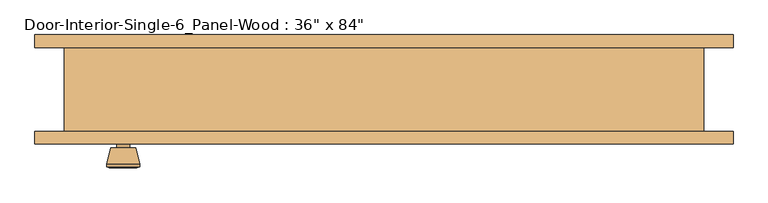
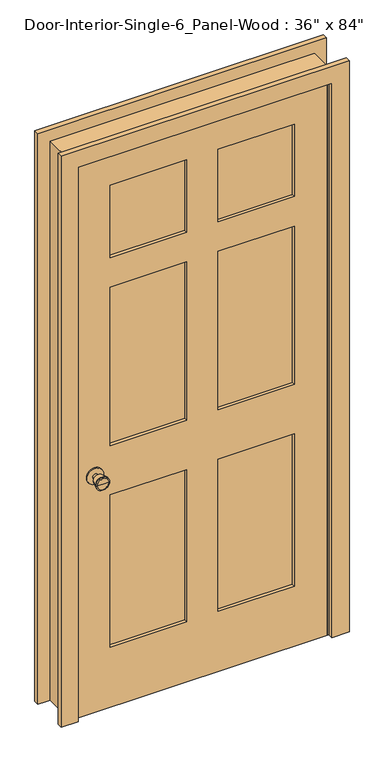
"""IFC4 building model written with IfcOpenShell, lengths in millimetres: door geometry."""

from ifc_helpers import new_model, si_unit, point, frame, frame_2d, origin, place, context, project, spatial, polyline, circle_curve, trimmed, segment, composite_curve, outline, extrude, faceted_brep, source, transform, mapped, element, save
from ifc_brep_helpers import plane_surface, cylinder_surface, revolved_surface, advanced_brep


def door_c610b25b(model_context):
    return source(origin(), model_context, "Body", "SolidModel", [
        advanced_brep(
        [(-393.7, -19.4, 914.4), (-403.7, -19.4, 914.4), (-383.7, -19.4, 914.4), (-373.2241324, 29.6, 914.4), (-414.1758676, 29.6, 914.4), (-393.7, 29.6, 914.4), (-368.7, 27.7721319, 914.4), (-418.7, 27.7721319, 914.4), (-368.7, 24.3084537, 914.4), (-418.7, 24.3084537, 914.4), (-375.063764, -0.4, 914.4), (-412.336236, -0.4, 914.4), (-383.7, -0.4, 914.4), (-403.7, -0.4, 914.4)],
        [
            (0, 1),
            (1, 2, circle_curve(frame((-393.7, -19.4, 914.4), z_axis=(0.0, -1.0, 0.0), x_axis=(-1.0, 0.0, 0.0)), 10.0)),
            (2, 0),
            (2, 1, circle_curve(frame((-393.7, -19.4, 914.4), z_axis=(0.0, -1.0, 0.0), x_axis=(-1.0, 0.0, 0.0)), 10.0)),
            (3, 4, circle_curve(frame((-393.7, 29.6, 914.4), z_axis=(0.0, 1.0, 0.0), x_axis=(-1.0, 0.0, 0.0)), 20.4758676)),
            (4, 5),
            (5, 3),
            (4, 3, circle_curve(frame((-393.7, 29.6, 914.4), z_axis=(0.0, 1.0, 0.0), x_axis=(-1.0, 0.0, 0.0)), 20.4758676)),
            (6, 7, circle_curve(frame((-393.7, 27.7721319, 914.4), z_axis=(0.0, 1.0, 0.0), x_axis=(-1.0, 0.0, 0.0)), 25.0)),
            (7, 4),
            (3, 6),
            (7, 6, circle_curve(frame((-393.7, 27.7721319, 914.4), z_axis=(0.0, 1.0, 0.0), x_axis=(-1.0, 0.0, 0.0)), 25.0)),
            (8, 9, circle_curve(frame((-393.7, 24.3084537, 914.4), z_axis=(0.0, 1.0, 0.0), x_axis=(-1.0, 0.0, 0.0)), 25.0)),
            (9, 7),
            (6, 8),
            (9, 8, circle_curve(frame((-393.7, 24.3084537, 914.4), z_axis=(0.0, 1.0, 0.0), x_axis=(-1.0, 0.0, 0.0)), 25.0)),
            (10, 11, circle_curve(frame((-393.7, -0.4, 914.4), z_axis=(0.0, 1.0, 0.0), x_axis=(-1.0, 0.0, 0.0)), 18.636236)),
            (11, 9),
            (8, 10),
            (11, 10, circle_curve(frame((-393.7, -0.4, 914.4), z_axis=(0.0, 1.0, 0.0), x_axis=(-1.0, 0.0, 0.0)), 18.636236)),
            (12, 13, circle_curve(frame((-393.7, -0.4, 914.4), z_axis=(0.0, 1.0, 0.0), x_axis=(-1.0, 0.0, 0.0)), 10.0)),
            (13, 11),
            (10, 12),
            (13, 12, circle_curve(frame((-393.7, -0.4, 914.4), z_axis=(0.0, 1.0, 0.0), x_axis=(-1.0, 0.0, 0.0)), 10.0)),
            (1, 13),
            (12, 2),
        ],
        [
            plane_surface(frame((-393.7, -19.4, 914.4), z_axis=(0.0, -1.0, 0.0), x_axis=(-1.0, 0.0, 0.0))),
            plane_surface(frame((-393.7, 29.6, 914.4), z_axis=(0.0, 1.0, 0.0), x_axis=(-1.0, 0.0, 0.0))),
            revolved_surface(polyline([(-414.1758676, 29.6, 914.4), (-418.7, 27.7721319, 914.4)]), (-393.7, -19.4, 914.4), (0.0, -1.0, 0.0)),
            cylinder_surface(frame((-393.7, -19.4, 914.4), z_axis=(0.0, -1.0, 0.0), x_axis=(-1.0, 0.0, 0.0)), 25.0),
            revolved_surface(polyline([(-418.7, 24.3084537, 914.4), (-412.336236, -0.4, 914.4)]), (-393.7, -19.4, 914.4), (0.0, -1.0, 0.0)),
            plane_surface(frame((-393.7, -0.4, 914.4), z_axis=(0.0, -1.0, 0.0), x_axis=(-1.0, 0.0, 0.0))),
            cylinder_surface(frame((-393.7, -19.4, 914.4), z_axis=(0.0, -1.0, 0.0), x_axis=(-1.0, 0.0, 0.0)), 10.0),
        ],
        [
            (0, [[1, 2, 3]]),
            (0, [[-3, 4, -1]]),
            (1, [[5, 6, 7]]),
            (1, [[8, -7, -6]]),
            (2, [[9, 10, -5, 11]]),
            (2, [[12, -11, -8, -10]]),
            (3, [[13, 14, -9, 15]]),
            (3, [[16, -15, -12, -14]]),
            (4, [[17, 18, -13, 19]]),
            (4, [[20, -19, -16, -18]]),
            (5, [[21, 22, -17, 23]]),
            (5, [[24, -23, -20, -22]]),
            (6, [[-2, 25, -21, 26]]),
            (6, [[-4, -26, -24, -25]]),
        ],
    ),
        extrude(outline(composite_curve([segment(trimmed(circle_curve(frame_2d((914.4, -393.7)), 30.0), [point((914.4, -423.7))], [point((914.4, -363.7))], False, "CARTESIAN"), True, "CONTINUOUS"), segment(trimmed(circle_curve(frame_2d((914.4, -393.7)), 30.0), [point((914.4, -363.7))], [point((914.4, -423.7))], False, "CARTESIAN"), True, "CONTINUOUS")], self_intersect=False)), frame((0.0, -25.4, 0.0), z_axis=(0.0, 1.0, 0.0), x_axis=(0.0, 0.0, 1.0)), (0.0, 0.0, 1.0), 6.0),
        advanced_brep(
        [(-393.7, -66.325, 914.4), (-383.7, -66.325, 914.4), (-403.7, -66.325, 914.4), (-373.2241324, -115.325, 914.4), (-393.7, -115.325, 914.4), (-414.1758676, -115.325, 914.4), (-368.7, -113.4971319, 914.4), (-418.7, -113.4971319, 914.4), (-368.7, -110.0334537, 914.4), (-418.7, -110.0334537, 914.4), (-375.063764, -85.325, 914.4), (-412.336236, -85.325, 914.4), (-383.7, -85.325, 914.4), (-403.7, -85.325, 914.4)],
        [
            (0, 1),
            (1, 2, circle_curve(frame((-393.7, -66.325, 914.4), z_axis=(0.0, 1.0, 0.0), x_axis=(-1.0, 0.0, 0.0)), 10.0)),
            (2, 0),
            (2, 1, circle_curve(frame((-393.7, -66.325, 914.4), z_axis=(0.0, 1.0, 0.0), x_axis=(-1.0, 0.0, 0.0)), 10.0)),
            (3, 4),
            (4, 5),
            (5, 3, circle_curve(frame((-393.7, -115.325, 914.4), z_axis=(0.0, -1.0, 0.0), x_axis=(-1.0, 0.0, 0.0)), 20.4758676)),
            (3, 5, circle_curve(frame((-393.7, -115.325, 914.4), z_axis=(0.0, -1.0, 0.0), x_axis=(-1.0, 0.0, 0.0)), 20.4758676)),
            (6, 3),
            (5, 7),
            (7, 6, circle_curve(frame((-393.7, -113.4971319, 914.4), z_axis=(0.0, -1.0, 0.0), x_axis=(-1.0, 0.0, 0.0)), 25.0)),
            (6, 7, circle_curve(frame((-393.7, -113.4971319, 914.4), z_axis=(0.0, -1.0, 0.0), x_axis=(-1.0, 0.0, 0.0)), 25.0)),
            (8, 6),
            (7, 9),
            (9, 8, circle_curve(frame((-393.7, -110.0334537, 914.4), z_axis=(0.0, -1.0, 0.0), x_axis=(-1.0, 0.0, 0.0)), 25.0)),
            (8, 9, circle_curve(frame((-393.7, -110.0334537, 914.4), z_axis=(0.0, -1.0, 0.0), x_axis=(-1.0, 0.0, 0.0)), 25.0)),
            (10, 8),
            (9, 11),
            (11, 10, circle_curve(frame((-393.7, -85.325, 914.4), z_axis=(0.0, -1.0, 0.0), x_axis=(-1.0, 0.0, 0.0)), 18.636236)),
            (10, 11, circle_curve(frame((-393.7, -85.325, 914.4), z_axis=(0.0, -1.0, 0.0), x_axis=(-1.0, 0.0, 0.0)), 18.636236)),
            (12, 10),
            (11, 13),
            (13, 12, circle_curve(frame((-393.7, -85.325, 914.4), z_axis=(0.0, -1.0, 0.0), x_axis=(-1.0, 0.0, 0.0)), 10.0)),
            (12, 13, circle_curve(frame((-393.7, -85.325, 914.4), z_axis=(0.0, -1.0, 0.0), x_axis=(-1.0, 0.0, 0.0)), 10.0)),
            (1, 12),
            (13, 2),
        ],
        [
            plane_surface(frame((-393.7, -66.325, 914.4), z_axis=(0.0, 1.0, 0.0), x_axis=(-1.0, 0.0, 0.0))),
            plane_surface(frame((-393.7, -115.325, 914.4), z_axis=(0.0, -1.0, 0.0), x_axis=(-1.0, 0.0, 0.0))),
            revolved_surface(polyline([(-414.1758676, -115.325, 914.4), (-418.7, -113.4971319, 914.4)]), (-393.7, -66.325, 914.4), (0.0, 1.0, 0.0)),
            cylinder_surface(frame((-393.7, -66.325, 914.4), z_axis=(0.0, 1.0, 0.0), x_axis=(-1.0, 0.0, 0.0)), 25.0),
            revolved_surface(polyline([(-418.7, -110.0334537, 914.4), (-412.336236, -85.325, 914.4)]), (-393.7, -66.325, 914.4), (0.0, 1.0, 0.0)),
            plane_surface(frame((-393.7, -85.325, 914.4), z_axis=(0.0, 1.0, 0.0), x_axis=(-1.0, 0.0, 0.0))),
            cylinder_surface(frame((-393.7, -66.325, 914.4), z_axis=(0.0, 1.0, 0.0), x_axis=(-1.0, 0.0, 0.0)), 10.0),
        ],
        [
            (0, [[1, 2, 3]]),
            (0, [[-3, 4, -1]]),
            (1, [[5, 6, 7]]),
            (1, [[-6, -5, 8]]),
            (2, [[9, -7, 10, 11]]),
            (2, [[-10, -8, -9, 12]]),
            (3, [[13, -11, 14, 15]]),
            (3, [[-14, -12, -13, 16]]),
            (4, [[17, -15, 18, 19]]),
            (4, [[-18, -16, -17, 20]]),
            (5, [[21, -19, 22, 23]]),
            (5, [[-22, -20, -21, 24]]),
            (6, [[25, -23, 26, -2]]),
            (6, [[-26, -24, -25, -4]]),
        ],
    ),
        extrude(outline(composite_curve([segment(trimmed(circle_curve(frame_2d((914.4, -393.7)), 30.0), [point((914.4, -423.7))], [point((914.4, -363.7))], False, "CARTESIAN"), True, "CONTINUOUS"), segment(trimmed(circle_curve(frame_2d((914.4, -393.7)), 30.0), [point((914.4, -363.7))], [point((914.4, -423.7))], False, "CARTESIAN"), True, "CONTINUOUS")], self_intersect=False)), frame((0.0, -66.325, 0.0), z_axis=(0.0, 1.0, 0.0), x_axis=(0.0, 0.0, 1.0)), (0.0, 0.0, 1.0), 6.0),
        faceted_brep([(482.6, -60.325, 0.0), (457.2, -60.325, 0.0), (457.2, -25.4, 0.0), (444.5, -25.4, 0.0), (444.5, 9.525, 0.0), (457.2, 9.525, 0.0), (457.2, 66.675, 0.0), (482.6, 66.675, 0.0), (482.6, 66.675, 2159.0), (482.6, -60.325, 2159.0), (457.2, 66.675, 2133.6), (-457.2, 66.675, 2133.6), (-457.2, 66.675, 0.0), (-482.6, 66.675, 0.0), (-482.6, 66.675, 2159.0), (457.2, 9.525, 2133.6), (444.5, 9.525, 2120.9), (-444.5, 9.525, 2120.9), (-444.5, 9.525, 0.0), (-457.2, 9.525, 0.0), (-457.2, 9.525, 2133.6), (444.5, -25.4, 2120.9), (457.2, -25.4, 2133.6), (-457.2, -25.4, 2133.6), (-457.2, -25.4, 0.0), (-444.5, -25.4, 0.0), (-444.5, -25.4, 2120.9), (457.2, -60.325, 2133.6), (-482.6, -60.325, 2159.0), (-482.6, -60.325, 0.0), (-457.2, -60.325, 0.0), (-457.2, -60.325, 2133.6)], [[[0, 1, 2, 3, 4, 5, 6, 7]], [[7, 8, 9, 0]], [[6, 10, 11, 12, 13, 14, 8, 7]], [[5, 15, 10, 6]], [[4, 16, 17, 18, 19, 20, 15, 5]], [[3, 21, 16, 4]], [[2, 22, 23, 24, 25, 26, 21, 3]], [[1, 27, 22, 2]], [[0, 9, 28, 29, 30, 31, 27, 1]], [[8, 14, 28, 9]], [[15, 20, 11, 10]], [[21, 26, 17, 16]], [[27, 31, 23, 22]], [[29, 13, 12, 19, 18, 25, 24, 30]], [[14, 13, 29, 28]], [[20, 19, 12, 11]], [[26, 25, 18, 17]], [[31, 30, 24, 23]]]),
        extrude(outline(polyline([(2133.6, -457.2), (0.0, -457.2), (0.0, 457.2), (2133.6, 457.2), (2133.6, -457.2)]), holes=[polyline([(2014.5375, 57.15), (2014.5375, 336.55), (1735.1375, 336.55), (1735.1375, 57.15), (2014.5375, 57.15)]), polyline([(1620.8375, 336.55), (1009.65, 336.55), (1009.65, 57.15), (1620.8375, 57.15), (1620.8375, 336.55)]), polyline([(1009.65, -57.15), (1009.65, -336.55), (1620.8375, -336.55), (1620.8375, -57.15), (1009.65, -57.15)]), polyline([(1735.1375, -336.55), (2014.5375, -336.55), (2014.5375, -57.15), (1735.1375, -57.15), (1735.1375, -336.55)]), polyline([(819.15, 57.15), (819.15, 336.55), (231.775, 336.55), (231.775, 57.15), (819.15, 57.15)]), polyline([(231.775, -57.15), (231.775, -336.55), (819.15, -336.55), (819.15, -57.15), (231.775, -57.15)])]), frame((0.0, -60.325, 0.0), z_axis=(0.0, 1.0, 0.0), x_axis=(0.0, 0.0, 1.0)), (0.0, 0.0, 1.0), 34.925),
        extrude(outline(polyline([(336.55, -37.0416667), (336.55, -48.6833333), (57.15, -48.6833333), (57.15, -37.0416667), (336.55, -37.0416667)])), frame((0.0, 0.0, 1735.1375), z_axis=(0.0, 0.0, 1.0), x_axis=(1.0, 0.0, 0.0)), (0.0, 0.0, 1.0), 279.4),
        extrude(outline(polyline([(336.55, -37.0416667), (336.55, -48.6833333), (57.15, -48.6833333), (57.15, -37.0416667), (336.55, -37.0416667)])), frame((0.0, 0.0, 1009.65), z_axis=(0.0, 0.0, 1.0), x_axis=(1.0, 0.0, 0.0)), (0.0, 0.0, 1.0), 611.1875),
        extrude(outline(polyline([(-57.15, -37.0416667), (-57.15, -48.6833333), (-336.55, -48.6833333), (-336.55, -37.0416667), (-57.15, -37.0416667)])), frame((0.0, 0.0, 1009.65), z_axis=(0.0, 0.0, 1.0), x_axis=(1.0, 0.0, 0.0)), (0.0, 0.0, 1.0), 611.1875),
        extrude(outline(polyline([(-57.15, -37.0416667), (-57.15, -48.6833333), (-336.55, -48.6833333), (-336.55, -37.0416667), (-57.15, -37.0416667)])), frame((0.0, 0.0, 1735.1375), z_axis=(0.0, 0.0, 1.0), x_axis=(1.0, 0.0, 0.0)), (0.0, 0.0, 1.0), 279.4),
        extrude(outline(polyline([(336.55, -37.0416667), (336.55, -48.6833333), (57.15, -48.6833333), (57.15, -37.0416667), (336.55, -37.0416667)])), frame((0.0, 0.0, 231.775), z_axis=(0.0, 0.0, 1.0), x_axis=(1.0, 0.0, 0.0)), (0.0, 0.0, 1.0), 587.375),
        extrude(outline(polyline([(-57.15, -37.0416667), (-57.15, -48.6833333), (-336.55, -48.6833333), (-336.55, -37.0416667), (-57.15, -37.0416667)])), frame((0.0, 0.0, 231.775), z_axis=(0.0, 0.0, 1.0), x_axis=(1.0, 0.0, 0.0)), (0.0, 0.0, 1.0), 587.375),
        extrude(outline(polyline([(0.0, 527.05), (2203.45, 527.05), (2203.45, -527.05), (0.0, -527.05), (0.0, -463.55), (2139.95, -463.55), (2139.95, 463.55), (0.0, 463.55), (0.0, 527.05)])), frame((0.0, -79.375, 0.0), z_axis=(0.0, 1.0, 0.0), x_axis=(0.0, 0.0, 1.0)), (0.0, 0.0, 1.0), 19.05),
        extrude(outline(polyline([(0.0, 527.05), (2203.45, 527.05), (2203.45, -527.05), (0.0, -527.05), (0.0, -463.55), (2139.95, -463.55), (2139.95, 463.55), (0.0, 463.55), (0.0, 527.05)])), frame((0.0, 66.675, 0.0), z_axis=(0.0, 1.0, 0.0), x_axis=(0.0, 0.0, 1.0)), (0.0, 0.0, 1.0), 19.05),
    ])


if __name__ == "__main__":
    model = new_model("IFC4")
    model_context = context("Model", 3, world=origin())
    ifc_project = project(units=[si_unit("LENGTHUNIT", "METRE", prefix="MILLI")], contexts=[model_context])
    site = spatial("IfcSite", under=ifc_project)
    building = spatial("IfcBuilding", under=site)
    placement = place(None, origin())
    door_shape = door_c610b25b(model_context)
    element("IfcDoor", 1, ObjectType="Door-Interior-Single-6_Panel-Wood : 36\" x 84\"", at=placement, inside=building, context=model_context, shape_type="MappedRepresentation", body=[
        mapped(door_shape, transform((0.0, 0.0, 0.0), x_axis=(1.0, 0.0, 0.0), y_axis=(0.0, 1.0, 0.0), z_axis=(0.0, 0.0, 1.0))),
    ])
    save(model, "model.ifc")

# Revit data of these elements
# Type "Door-Interior-Single-6_Panel-Wood : 36\" x 84\""
#   Type Mark = "12"
#   Assembly Code = "C1020300"
#   Analytic Construction = "Wooden"
#   Top Rail = 0' - 4 11/16"
#   Top Panel = 0' - 11"
#   Thickness = 0' - 1 3/8"
#   Thermal Resistance (R) = 2.5876 (h·ft²·°F)/BTU
#   Swing Angle [instance default] = 90.00°
#   Stiles = 0' - 4 3/4"
#   Rough Width = 3' - 2"
#   Rough Height = 7' - 1"
#   Mullion = 0' - 4 1/2"
#   Lock Rail = 0' - 7 1/2"
#   Intermediate Rail = 0' - 4 1/2"
#   Height = 7' - 0"
#   Width = 3' - 0"
#   Heat Transfer Coefficient (U) = 0.3865 BTU/(h·ft²·°F)
#   Bottom Rail = 0' - 9 1/8"
#   Trim Material = Cherry
#   Panel Material = Cherry
#   Frame Material = Cherry
#   Door Handle Material = Aluminum
#   Visual Light Transmittance = 0
#   Solar Heat Gain Coefficient = 0
#   Wall Closure = (empty or 0)
#   Function = (empty or 0)
# Element 1 (IfcDoor, "Door-Interior-Single-6_Panel-Wood : 36\" x 84\"")
#   Materials on its faces: "Cherry", "Aluminum"
# Materials
#   "Cherry": class "Wood", colour RGB 226 177 128, transparency 0, Description = "Prunus Serotina", Cost = 0
#   "Aluminum": class "Metal", colour RGB 247 247 247, transparency 0, Description = "Aluminum 6061", Cost = 0
